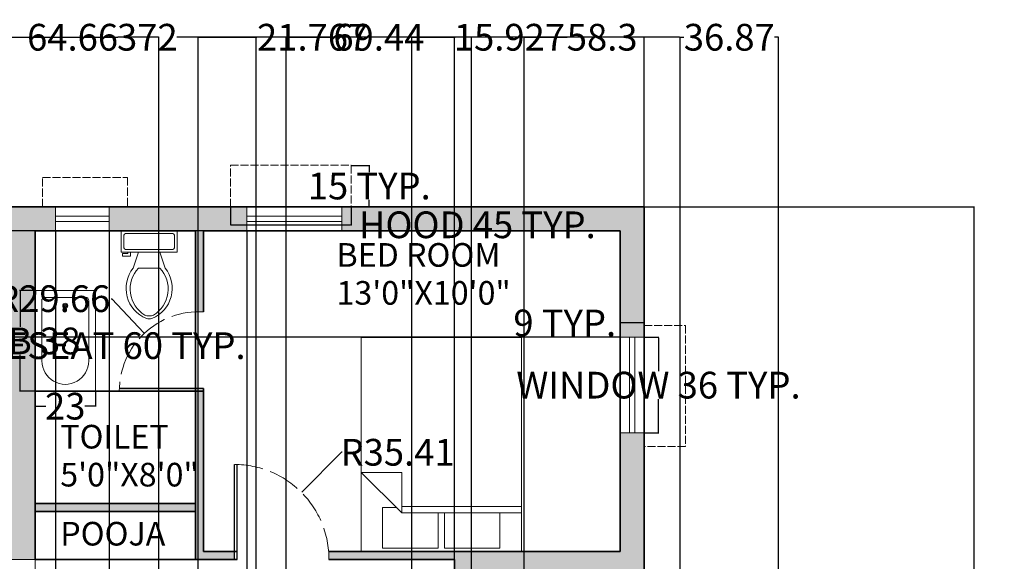
# Model space of a CAD drawing. Units: inches. Extents: x 300 to 1007, y 2 to 1069.
# Tile 12 of 12: x 617 to 986, y 867 to 1069. Entities that reach past the tile are written whole.
import ezdxf

# ---------------------------------------------------------------- set-up
doc = ezdxf.new("R2010")
doc.units = ezdxf.units.IN
doc.header["$MEASUREMENT"] = 0
doc.linetypes.add('ACAD_ISO02W100', pattern=[15, 12, -3])
for name, color, linetype, lineweight in [('A-ANNO-DIMS', 2, 'Continuous', 18), ('A-AREA-IDEN', 7, 'Continuous', 18), ('A-DOOR', 3, 'Continuous', 25), ('A-DOOR-SWNG', 3, 'ACAD_ISO02W100', 13), ('A-FLOR-FIXT', 9, 'Continuous', 18), ('A-FURN', 8, 'Continuous', 18), ('A-GLAZ', 4, 'Continuous', 18), ('A-GLAZ-OVHD', 8, 'ACAD_ISO02W100', 13), ('A-WALL', 7, 'Continuous', 35), ('A-WALL-OVHD', 8, 'ACAD_ISO02W100', 18)]:
    doc.layers.add(name, color=color, linetype=linetype, lineweight=lineweight)
doc.layers.add('A-WALL-PATT', color=9, linetype='Continuous', lineweight=9, true_color=0xc7c8ca)
doc.styles.get("Standard").update_dxf_attribs({"font": 'arial.ttf'})
doc.dimstyles.get("Standard").update_dxf_attribs({"dimtxt": 10, "dimasz": 0.18, "dimexe": 0.18, "dimexo": 0.0625, "dimgap": 0.09, "dimtad": 0, "dimtih": 1, "dimtoh": 1, "dimdec": 0, "dimzin": 0, "dimdsep": 46, "dimlunit": 3, "dimtxsty": 'Standard', "dimcen": 0.09, "dimadec": 0, "dimazin": 0, "dimtfac": 1, "dimtdec": 0, "dimtofl": 0, "dimtmove": 0, "dimatfit": 3, "dimfxl": 1, "dimtolj": 1, "dimtzin": 0, "dimarcsym": 0})

# ---------------------------------------------------------------- blocks, each defined once
blk = doc.blocks.new('Bath Tub - 26 x 60 in.')
for p, q in [((9, -17), (9, -19)), ((8, -18), (10, -18))]:
    blk.add_line(p, q)
blk.add_lwpolyline([(0, -36), (0, 0), (60, 0), (60, -36)], close=True)
for points in [[(6, -4), (42, -4)], [(4, -30), (4, -6)], [(42, -32), (6, -32)]]:
    blk.add_lwpolyline(points)
for radius in [1.5, 1]:
    blk.add_circle((9, -18), radius)
for centre, radius, start, end in [((5.75, -5.75), 1.77, 81.8699, 188.1301), ((42, -18), 14, 270, 90), ((5.75, -30.25), 1.77, 171.8699, 278.1301)]:
    blk.add_arc(centre, radius, start, end)
blk = doc.blocks.new('Toilet - top')
for p, q in [((9.5, -6), (9.5, -2)), ((-10, -8.5), (-8, -8.5)), ((-10, -9.5), (-10, -8.5)), ((-7, -9.5), (-10, -9.5)), ((-8, -8.5), (-8, -8)), ((-7, -8), (-7, -9.5)), ((-4, -8), (-6, -14)), ((4, -8), (6, -14)), ((4, -14), (-4, -14))]:
    blk.add_line(p, q)
blk.add_lwpolyline([(10.5, -8), (10.5, 0), (-10.5, 0), (-10.5, -8)], close=True)
for points in [[(-9.5, -2), (-9.5, -6)], [(8.5, -1), (-8.5, -1)], [(-8.5, -7), (8.5, -7)]]:
    blk.add_lwpolyline(points)
for centre, radius, start, end in [((-8.62, -1.88), 0.884, 81.8699, 188.1301), ((8.62, -1.88), 0.884, 351.8699, 98.1301), ((-8.62, -6.12), 0.884, 171.8699, 278.1301), ((8.62, -6.12), 0.884, 261.8699, 8.1301), ((3.52, -21.58), 12.17, 141.4691, 247.9714), ((4.2, -21.82), 11.33, 136.3677, 238.9468), ((-3.52, -21.58), 12.17, 292.0284, 38.5307), ((-4.2, -21.82), 11.33, 301.053, 43.6321), ((0, -27.88), 4, 245.7318, 294.2682), ((0, -29), 4, 254.8605, 285.1395)]:
    blk.add_arc(centre, radius, start, end)
blk = doc.blocks.new('Bed - Queen')
for p, q in [((0, -80.00003), (0, 0)), ((0, 0), (59.99999, 0)), ((59.99999, 0), (59.99999, -80.00003)), ((7.99999, -1.2), (28.79998, -1.2)), ((7.99999, -14.4), (7.99999, -1.2)), ((28.79998, -1.2), (28.79998, -14.4)), ((31.19999, -1.2), (51.99999, -1.2)), ((31.19999, -14.4), (31.19999, -1.2)), ((51.99999, -1.2), (51.99999, -16.4)), ((0, -14.4), (44.8, -14.4)), ((59.99999, -29.6), (44.8, -14.4)), ((44.8, -14.4), (44.8, -29.6)), ((44.8, -16.8), (0, -16.8)), ((51.99999, -16.4), (46.79936, -16.4)), ((44.8, -29.6), (59.99999, -29.6)), ((59.99999, -80.00003), (0, -80.00003))]:
    blk.add_line(p, q)
blk = doc.blocks.new('WIN-36')
for p, q in [((-36, -4.5), (-36, 4.5)), ((0, -4.5), (0, 4.5)), ((0, 1), (-36, 1)), ((-36, 0), (-36, -4.5)), ((0, -1), (-36, -1))]:
    blk.add_line(p, q)
blk = doc.blocks.new('WIN-35_1-2')
for p, q in [((0, -4.5), (0, 4.5)), ((35.5, 0), (35.5, 4.5)), ((35.5, 4.5), (35.5, -4.5)), ((0, 1), (35.5, 1)), ((0, -1), (35.5, -1))]:
    blk.add_line(p, q)
blk = doc.blocks.new('WINDOW-HOOD-45')
at = {"ltscale": 0.25}
for p, q in [((0, 0), (0, 15.48)), ((0, 15.48), (45.18, 15.48)), ((45.18, 15.48), (45.18, 0))]:
    blk.add_line(p, q, dxfattribs=at)
blk = doc.blocks.new('*D39')
at = {"layer": 'A-ANNO-DIMS', "color": 0, "lineweight": -2, "transparency": 16777216}
for p, q in [((622.76, 968.04), (617.01, 968.04)), ((617.19, 967.86), (617.19, 954.44)), ((617.19, 930.63), (617.19, 944.04)), ((622.76, 930.45), (617.01, 930.45))]:
    blk.add_line(p, q, dxfattribs=at)
at = {"layer": 'A-ANNO-DIMS', "color": 0, "transparency": 16777216}
for points in [[(617.16, 967.86), (617.22, 967.86), (617.19, 968.04)], [(617.16, 930.63), (617.22, 930.63), (617.19, 930.45)]]:
    blk.add_solid(points, dxfattribs=at)
at = {"layer": 'Defpoints', "color": 0, "transparency": 16777216}
for p in [(622.83, 968.04), (617.19, 930.45), (622.83, 930.45)]:
    blk.add_point(p, dxfattribs=at)
at = {"layer": 'A-ANNO-DIMS', "color": 0, "transparency": 16777216, "insert": (617.19, 949.24), "char_height": 10, "attachment_point": 5}
blk.add_mtext('\\A1;TUB 38', dxfattribs=at)
blk = doc.blocks.new('*D40')
at = {"layer": 'A-ANNO-DIMS', "color": 0, "lineweight": -2, "transparency": 16777216}
for p, q in [((622.83, 930.38), (622.83, 924.63)), ((645.38, 930.38), (645.38, 924.63)), ((623.01, 924.81), (626.77, 924.81)), ((645.2, 924.81), (641.44, 924.81))]:
    blk.add_line(p, q, dxfattribs=at)
at = {"layer": 'A-ANNO-DIMS', "color": 0, "transparency": 16777216}
for points in [[(623.01, 924.84), (623.01, 924.78), (622.83, 924.81)], [(645.2, 924.84), (645.2, 924.78), (645.38, 924.81)]]:
    blk.add_solid(points, dxfattribs=at)
at = {"layer": 'Defpoints', "color": 0, "transparency": 16777216}
for p in [(622.83, 930.45), (645.38, 930.45), (645.38, 924.81)]:
    blk.add_point(p, dxfattribs=at)
at = {"layer": 'A-ANNO-DIMS', "color": 0, "transparency": 16777216, "insert": (634.1, 924.81), "char_height": 10, "attachment_point": 5}
blk.add_mtext('\\A1;23', dxfattribs=at)
blk = doc.blocks.new('*D45')
at = {"layer": 'A-ANNO-DIMS', "color": 0, "lineweight": -2, "transparency": 16777216}
for p, q in [((850.89, 950.57), (856.37, 950.57)), ((856.19, 950.39), (856.19, 937.94)), ((856.19, 914.97), (856.19, 927.41)), ((850.89, 914.79), (856.37, 914.79))]:
    blk.add_line(p, q, dxfattribs=at)
at = {"layer": 'A-ANNO-DIMS', "color": 0, "transparency": 16777216}
for points in [[(856.16, 950.39), (856.22, 950.39), (856.19, 950.57)], [(856.16, 914.97), (856.22, 914.97), (856.19, 914.79)]]:
    blk.add_solid(points, dxfattribs=at)
at = {"layer": 'Defpoints', "color": 0, "transparency": 16777216}
for p in [(850.83, 950.57), (856.19, 950.57), (850.83, 914.79)]:
    blk.add_point(p, dxfattribs=at)
at = {"layer": 'A-ANNO-DIMS', "color": 0, "transparency": 16777216, "insert": (856.19, 932.68), "char_height": 10, "attachment_point": 5}
blk.add_mtext('\\A1;WINDOW 36 TYP.', dxfattribs=at)
blk = doc.blocks.new('*D46')
at = {"layer": 'A-ANNO-DIMS', "color": 0, "lineweight": -2, "transparency": 16777216}
for p, q in [((841.83, 955.94), (841.65, 955.94)), ((841.83, 950.63), (841.83, 956.12)), ((850.65, 955.94), (842.01, 955.94)), ((850.83, 950.63), (850.83, 956.12))]:
    blk.add_line(p, q, dxfattribs=at)
at = {"layer": 'A-ANNO-DIMS', "color": 0, "transparency": 16777216}
for points in [[(842.01, 955.97), (842.01, 955.91), (841.83, 955.94)], [(850.65, 955.97), (850.65, 955.91), (850.83, 955.94)]]:
    blk.add_solid(points, dxfattribs=at)
at = {"layer": 'Defpoints', "color": 0, "transparency": 16777216}
for p in [(841.83, 955.94), (841.83, 950.57), (850.83, 950.57)]:
    blk.add_point(p, dxfattribs=at)
at = {"layer": 'A-ANNO-DIMS', "color": 0, "transparency": 16777216, "insert": (821.1, 955.94), "char_height": 10, "attachment_point": 5}
blk.add_mtext('\\A1;9 TYP.', dxfattribs=at)
blk = doc.blocks.new('*D47')
at = {"layer": 'A-ANNO-DIMS', "color": 0, "lineweight": -2, "transparency": 16777216}
for p, q in [((695.95, 999.38), (695.95, 992.49)), ((741.12, 999.38), (741.12, 992.49)), ((696.13, 992.67), (740.94, 992.67)), ((741.12, 992.67), (741.3, 992.67))]:
    blk.add_line(p, q, dxfattribs=at)
at = {"layer": 'A-ANNO-DIMS', "color": 0, "transparency": 16777216}
for points in [[(696.13, 992.7), (696.13, 992.64), (695.95, 992.67)], [(740.94, 992.7), (740.94, 992.64), (741.12, 992.67)]]:
    blk.add_solid(points, dxfattribs=at)
at = {"layer": 'Defpoints', "color": 0, "transparency": 16777216}
for p in [(695.95, 999.45), (741.12, 999.45), (741.12, 992.67)]:
    blk.add_point(p, dxfattribs=at)
at = {"layer": 'A-ANNO-DIMS', "color": 0, "transparency": 16777216, "insert": (788.36, 992.67), "char_height": 10, "attachment_point": 5}
blk.add_mtext('\\A1;HOOD 45 TYP.', dxfattribs=at)
blk = doc.blocks.new('*D48')
at = {"layer": 'A-ANNO-DIMS', "color": 0, "lineweight": -2, "transparency": 16777216}
for p, q in [((741.19, 1014.92), (748.08, 1014.92)), ((747.9, 1014.74), (747.9, 1012.38)), ((741.19, 999.45), (748.08, 999.45)), ((747.9, 999.63), (747.9, 1001.99))]:
    blk.add_line(p, q, dxfattribs=at)
at = {"layer": 'A-ANNO-DIMS', "color": 0, "transparency": 16777216}
for points in [[(747.87, 1014.74), (747.93, 1014.74), (747.9, 1014.92)], [(747.87, 999.63), (747.93, 999.63), (747.9, 999.45)]]:
    blk.add_solid(points, dxfattribs=at)
at = {"layer": 'Defpoints', "color": 0, "transparency": 16777216}
for p in [(741.12, 1014.92), (747.9, 1014.92), (741.12, 999.45)]:
    blk.add_point(p, dxfattribs=at)
at = {"layer": 'A-ANNO-DIMS', "color": 0, "transparency": 16777216, "insert": (747.9, 1007.18), "char_height": 10, "attachment_point": 5}
blk.add_mtext('\\A1;15 TYP.', dxfattribs=at)
blk = doc.blocks.new('*D49')
at = {"layer": 'A-ANNO-DIMS', "color": 0, "lineweight": -2, "transparency": 16777216}
for p, q in [((520.83, 956.38), (520.83, 947.27)), ((580.83, 956.38), (580.83, 947.27)), ((521.01, 947.45), (580.65, 947.45)), ((580.83, 947.45), (581.01, 947.45))]:
    blk.add_line(p, q, dxfattribs=at)
at = {"layer": 'A-ANNO-DIMS', "color": 0, "transparency": 16777216}
for points in [[(521.01, 947.48), (521.01, 947.42), (520.83, 947.45)], [(580.65, 947.48), (580.65, 947.42), (580.83, 947.45)]]:
    blk.add_solid(points, dxfattribs=at)
at = {"layer": 'Defpoints', "color": 0, "transparency": 16777216}
for p in [(520.83, 956.45), (580.83, 956.45), (580.83, 947.45)]:
    blk.add_point(p, dxfattribs=at)
at = {"layer": 'A-ANNO-DIMS', "color": 0, "transparency": 16777216, "insert": (644.03, 947.45), "char_height": 10, "attachment_point": 5}
blk.add_mtext('\\A1;LOVESEAT 60 TYP.', dxfattribs=at)
blk = doc.blocks.new('*D75')
at = {"layer": 'A-ANNO-DIMS', "color": 0, "lineweight": -2, "transparency": 16777216}
for p, q in [((478.83, 999.51), (478.83, 1063.03)), ((479.01, 1062.85), (653.74, 1062.85)), ((850.65, 1062.85), (675.91, 1062.85)), ((850.83, 999.51), (850.83, 1063.03))]:
    blk.add_line(p, q, dxfattribs=at)
at = {"layer": 'A-ANNO-DIMS', "color": 0, "transparency": 16777216}
for points in [[(479.01, 1062.88), (479.01, 1062.82), (478.83, 1062.85)], [(850.65, 1062.88), (850.65, 1062.82), (850.83, 1062.85)]]:
    blk.add_solid(points, dxfattribs=at)
at = {"layer": 'Defpoints', "color": 0, "transparency": 16777216}
for p in [(850.83, 1062.85), (478.83, 999.45), (850.83, 999.45)]:
    blk.add_point(p, dxfattribs=at)
at = {"layer": 'A-ANNO-DIMS', "color": 0, "transparency": 16777216, "insert": (664.83, 1062.85), "char_height": 10, "attachment_point": 5}
blk.add_mtext('\\A1;372', dxfattribs=at)
blk = doc.blocks.new('*D78')
at = {"layer": 'A-ANNO-DIMS', "color": 0, "lineweight": -2, "transparency": 16777216}
for p, q in [((850.89, 999.45), (974.48, 999.45)), ((974.3, 999.27), (974.3, 809.65)), ((974.3, 609.63), (974.3, 799.25)), ((841.89, 609.45), (974.48, 609.45))]:
    blk.add_line(p, q, dxfattribs=at)
at = {"layer": 'A-ANNO-DIMS', "color": 0, "transparency": 16777216}
for points in [[(974.27, 999.27), (974.33, 999.27), (974.3, 999.45)], [(974.27, 609.63), (974.33, 609.63), (974.3, 609.45)]]:
    blk.add_solid(points, dxfattribs=at)
at = {"layer": 'Defpoints', "color": 0, "transparency": 16777216}
for p in [(850.83, 999.45), (974.3, 999.45), (841.83, 609.45)]:
    blk.add_point(p, dxfattribs=at)
at = {"layer": 'A-ANNO-DIMS', "color": 0, "transparency": 16777216, "insert": (974.3, 804.45), "char_height": 10, "attachment_point": 5}
blk.add_mtext('\\A1;390', dxfattribs=at)
blk = doc.blocks.new('*D80')
at = {"layer": 'A-ANNO-DIMS', "color": 0, "lineweight": -2, "transparency": 16777216}
for p, q in [((683.83, 717.31), (683.83, 1063.03)), ((684.01, 1062.85), (705.41, 1062.85)), ((705.59, 717.31), (705.59, 1063.03)), ((705.59, 1062.85), (705.77, 1062.85))]:
    blk.add_line(p, q, dxfattribs=at)
at = {"layer": 'A-ANNO-DIMS', "color": 0, "transparency": 16777216}
for points in [[(684.01, 1062.88), (684.01, 1062.82), (683.83, 1062.85)], [(705.41, 1062.88), (705.41, 1062.82), (705.59, 1062.85)]]:
    blk.add_solid(points, dxfattribs=at)
at = {"layer": 'Defpoints', "color": 0, "transparency": 16777216}
for p in [(705.59, 1062.85), (683.83, 717.25), (705.59, 717.25)]:
    blk.add_point(p, dxfattribs=at)
at = {"layer": 'A-ANNO-DIMS', "color": 0, "transparency": 16777216, "insert": (726.71, 1062.85), "char_height": 10, "attachment_point": 5}
blk.add_mtext('\\A1;21.767', dxfattribs=at)
blk = doc.blocks.new('*D82')
at = {"layer": 'A-ANNO-DIMS', "color": 0, "lineweight": -2, "transparency": 16777216}
for p, q in [((763.9, 700.01), (763.9, 1063.03)), ((764.08, 1062.85), (779.65, 1062.85)), ((779.83, 700.01), (779.83, 1063.03)), ((779.83, 1062.85), (780.01, 1062.85))]:
    blk.add_line(p, q, dxfattribs=at)
at = {"layer": 'A-ANNO-DIMS', "color": 0, "transparency": 16777216}
for points in [[(764.08, 1062.88), (764.08, 1062.82), (763.9, 1062.85)], [(779.65, 1062.88), (779.65, 1062.82), (779.83, 1062.85)]]:
    blk.add_solid(points, dxfattribs=at)
at = {"layer": 'Defpoints', "color": 0, "transparency": 16777216}
for p in [(779.83, 1062.85), (763.9, 699.95), (779.83, 699.95)]:
    blk.add_point(p, dxfattribs=at)
at = {"layer": 'A-ANNO-DIMS', "color": 0, "transparency": 16777216, "insert": (800.38, 1062.85), "char_height": 10, "attachment_point": 5}
blk.add_mtext('\\A1;15.927', dxfattribs=at)
blk = doc.blocks.new('*D84')
at = {"layer": 'A-ANNO-DIMS', "color": 0, "lineweight": -2, "transparency": 16777216}
for p, q in [((864.25, 225.89), (864.25, 1063.03)), ((864.43, 1062.85), (865.73, 1062.85)), ((900.94, 1062.85), (899.65, 1062.85)), ((901.12, 225.89), (901.12, 1063.03))]:
    blk.add_line(p, q, dxfattribs=at)
at = {"layer": 'A-ANNO-DIMS', "color": 0, "transparency": 16777216}
for points in [[(864.43, 1062.88), (864.43, 1062.82), (864.25, 1062.85)], [(900.94, 1062.88), (900.94, 1062.82), (901.12, 1062.85)]]:
    blk.add_solid(points, dxfattribs=at)
at = {"layer": 'Defpoints', "color": 0, "transparency": 16777216}
for p in [(901.12, 1062.85), (864.25, 225.83), (901.12, 225.83)]:
    blk.add_point(p, dxfattribs=at)
at = {"layer": 'A-ANNO-DIMS', "color": 0, "transparency": 16777216, "insert": (882.69, 1062.85), "char_height": 10, "attachment_point": 5}
blk.add_mtext('\\A1;36.87', dxfattribs=at)
blk = doc.blocks.new('*D86')
at = {"layer": 'A-ANNO-DIMS', "color": 0, "lineweight": -2, "transparency": 16777216}
for p, q in [((805.95, 235.15), (805.95, 1063.03)), ((806.13, 1062.85), (822.02, 1062.85)), ((864.07, 1062.85), (848.18, 1062.85)), ((864.25, 235.15), (864.25, 1063.03))]:
    blk.add_line(p, q, dxfattribs=at)
at = {"layer": 'A-ANNO-DIMS', "color": 0, "transparency": 16777216}
for points in [[(806.13, 1062.88), (806.13, 1062.82), (805.95, 1062.85)], [(864.07, 1062.88), (864.07, 1062.82), (864.25, 1062.85)]]:
    blk.add_solid(points, dxfattribs=at)
at = {"layer": 'Defpoints', "color": 0, "transparency": 16777216}
for p in [(864.25, 1062.85), (805.95, 235.08), (864.25, 235.08)]:
    blk.add_point(p, dxfattribs=at)
at = {"layer": 'A-ANNO-DIMS', "color": 0, "transparency": 16777216, "insert": (835.1, 1062.85), "char_height": 10, "attachment_point": 5}
blk.add_mtext('\\A1;58.3', dxfattribs=at)
blk = doc.blocks.new('*D94')
at = {"layer": 'A-ANNO-DIMS', "color": 0, "lineweight": -2, "transparency": 16777216}
for p, q in [((841.76, 990.45), (354.19, 990.45)), ((354.37, 990.27), (354.37, 975.71)), ((354.37, 950.75), (354.37, 965.31)), ((841.76, 950.57), (354.19, 950.57))]:
    blk.add_line(p, q, dxfattribs=at)
at = {"layer": 'A-ANNO-DIMS', "color": 0, "transparency": 16777216}
for points in [[(354.34, 990.27), (354.4, 990.27), (354.37, 990.45)], [(354.34, 950.75), (354.4, 950.75), (354.37, 950.57)]]:
    blk.add_solid(points, dxfattribs=at)
at = {"layer": 'Defpoints', "color": 0, "transparency": 16777216}
for p in [(354.37, 990.45), (841.83, 990.45), (841.83, 950.57)]:
    blk.add_point(p, dxfattribs=at)
at = {"layer": 'A-ANNO-DIMS', "color": 0, "transparency": 16777216, "insert": (354.37, 970.51), "char_height": 10, "attachment_point": 5}
blk.add_mtext('\\A1;39.88', dxfattribs=at)
blk = doc.blocks.new('*D99')
at = {"layer": 'A-ANNO-DIMS', "color": 0, "lineweight": -2, "transparency": 16777216}
for p, q in [((604.49, 482.45), (604.49, 1063.03)), ((604.67, 1062.85), (619.83, 1062.85)), ((668.97, 1062.85), (653.8, 1062.85)), ((669.15, 482.45), (669.15, 1063.03))]:
    blk.add_line(p, q, dxfattribs=at)
at = {"layer": 'A-ANNO-DIMS', "color": 0, "transparency": 16777216}
for points in [[(604.67, 1062.88), (604.67, 1062.82), (604.49, 1062.85)], [(668.97, 1062.88), (668.97, 1062.82), (669.15, 1062.85)]]:
    blk.add_solid(points, dxfattribs=at)
at = {"layer": 'Defpoints', "color": 0, "transparency": 16777216}
for p in [(669.15, 1062.85), (604.49, 482.38), (669.15, 482.38)]:
    blk.add_point(p, dxfattribs=at)
at = {"layer": 'A-ANNO-DIMS', "color": 0, "transparency": 16777216, "insert": (636.82, 1062.85), "char_height": 10, "attachment_point": 5}
blk.add_mtext('\\A1;64.66', dxfattribs=at)
blk = doc.blocks.new('*D100')
at = {"layer": 'A-ANNO-DIMS', "color": 0, "lineweight": -2, "transparency": 16777216}
for p, q in [((716.78, 482.45), (716.78, 1063.03)), ((716.96, 1062.85), (734.53, 1062.85)), ((786.04, 1062.85), (768.47, 1062.85)), ((786.22, 482.45), (786.22, 1063.03))]:
    blk.add_line(p, q, dxfattribs=at)
at = {"layer": 'A-ANNO-DIMS', "color": 0, "transparency": 16777216}
for points in [[(716.96, 1062.88), (716.96, 1062.82), (716.78, 1062.85)], [(786.04, 1062.88), (786.04, 1062.82), (786.22, 1062.85)]]:
    blk.add_solid(points, dxfattribs=at)
at = {"layer": 'Defpoints', "color": 0, "transparency": 16777216}
for p in [(786.22, 1062.85), (716.78, 482.38), (786.22, 482.38)]:
    blk.add_point(p, dxfattribs=at)
at = {"layer": 'A-ANNO-DIMS', "color": 0, "transparency": 16777216, "insert": (751.5, 1062.85), "char_height": 10, "attachment_point": 5}
blk.add_mtext('\\A1;69.44', dxfattribs=at)
blk = doc.blocks.new('*D106')
at = {"layer": 'A-ANNO-DIMS', "color": 0, "lineweight": -2, "transparency": 16777216}
for p, q in [((582.11, 990.38), (582.11, 8.45)), ((630.49, 990.38), (630.49, 8.45)), ((582.29, 8.63), (589.12, 8.63)), ((630.31, 8.63), (623.47, 8.63))]:
    blk.add_line(p, q, dxfattribs=at)
at = {"layer": 'A-ANNO-DIMS', "color": 0, "transparency": 16777216}
for points in [[(582.29, 8.66), (582.29, 8.6), (582.11, 8.63)], [(630.31, 8.66), (630.31, 8.6), (630.49, 8.63)]]:
    blk.add_solid(points, dxfattribs=at)
at = {"layer": 'Defpoints', "color": 0, "transparency": 16777216}
for p in [(582.11, 990.45), (630.49, 990.45), (630.49, 8.63)]:
    blk.add_point(p, dxfattribs=at)
at = {"layer": 'A-ANNO-DIMS', "color": 0, "transparency": 16777216, "insert": (606.3, 8.63), "char_height": 10, "attachment_point": 5}
blk.add_mtext('\\A1;48.38', dxfattribs=at)
blk = doc.blocks.new('*D107')
at = {"layer": 'A-ANNO-DIMS', "color": 0, "lineweight": -2, "transparency": 16777216}
for p, q in [((630.49, 990.38), (630.49, 8.45)), ((650.47, 990.38), (650.47, 8.45)), ((630.67, 8.63), (650.29, 8.63)), ((650.47, 8.63), (650.65, 8.63))]:
    blk.add_line(p, q, dxfattribs=at)
at = {"layer": 'A-ANNO-DIMS', "color": 0, "transparency": 16777216}
for points in [[(630.67, 8.66), (630.67, 8.6), (630.49, 8.63)], [(650.29, 8.66), (650.29, 8.6), (650.47, 8.63)]]:
    blk.add_solid(points, dxfattribs=at)
at = {"layer": 'Defpoints', "color": 0, "transparency": 16777216}
for p in [(630.49, 990.45), (650.47, 990.45), (650.47, 8.63)]:
    blk.add_point(p, dxfattribs=at)
at = {"layer": 'A-ANNO-DIMS', "color": 0, "transparency": 16777216, "insert": (667.15, 8.63), "char_height": 10, "attachment_point": 5}
blk.add_mtext('\\A1;19.98', dxfattribs=at)
blk = doc.blocks.new('*D108')
at = {"layer": 'A-ANNO-DIMS', "color": 0, "lineweight": -2, "transparency": 16777216}
for p, q in [((650.47, 990.38), (650.47, 8.45)), ((702.09, 990.38), (702.09, 8.45)), ((650.65, 8.63), (659.37, 8.63)), ((701.91, 8.63), (693.19, 8.63))]:
    blk.add_line(p, q, dxfattribs=at)
at = {"layer": 'A-ANNO-DIMS', "color": 0, "transparency": 16777216}
for points in [[(650.65, 8.66), (650.65, 8.6), (650.47, 8.63)], [(701.91, 8.66), (701.91, 8.6), (702.09, 8.63)]]:
    blk.add_solid(points, dxfattribs=at)
at = {"layer": 'Defpoints', "color": 0, "transparency": 16777216}
for p in [(650.47, 990.45), (702.09, 990.45), (702.09, 8.63)]:
    blk.add_point(p, dxfattribs=at)
at = {"layer": 'A-ANNO-DIMS', "color": 0, "transparency": 16777216, "insert": (676.28, 8.63), "char_height": 10, "attachment_point": 5}
blk.add_mtext('\\A1;51.62', dxfattribs=at)
blk = doc.blocks.new('*D114')
at = {"layer": 'A-ANNO-DIMS', "color": 0, "lineweight": -2, "transparency": 16777216}
for p, q in [((737.55, 907.56), (722.63, 892.69)), ((737.73, 907.56), (737.55, 907.56)), ((697.33, 867.57), (697.51, 867.57)), ((697.42, 867.48), (697.42, 867.66))]:
    blk.add_line(p, q, dxfattribs=at)
at = {"layer": 'A-ANNO-DIMS', "color": 0, "transparency": 16777216}
blk.add_solid([(722.61, 892.71), (722.65, 892.67), (722.5, 892.57)], dxfattribs=at)
at = {"layer": 'Defpoints', "color": 0, "transparency": 16777216}
for p in [(722.5, 892.57), (697.42, 867.57)]:
    blk.add_point(p, dxfattribs=at)
at = {"layer": 'A-ANNO-DIMS', "color": 0, "transparency": 16777216, "insert": (758.51, 907.56), "char_height": 10, "attachment_point": 5}
blk.add_mtext('\\A1;R35.41', dxfattribs=at)
blk = doc.blocks.new('*D118')
at = {"layer": 'A-ANNO-DIMS', "color": 0, "lineweight": -2, "transparency": 16777216}
for p, q in [((651.31, 965.03), (651.49, 965.03)), ((651.49, 965.03), (663.55, 952.19)), ((683.9, 930.45), (684.08, 930.45)), ((683.99, 930.36), (683.99, 930.54))]:
    blk.add_line(p, q, dxfattribs=at)
at = {"layer": 'A-ANNO-DIMS', "color": 0, "transparency": 16777216}
blk.add_solid([(663.57, 952.21), (663.53, 952.17), (663.68, 952.06)], dxfattribs=at)
at = {"layer": 'Defpoints', "color": 0, "transparency": 16777216}
for p in [(663.68, 952.06), (683.99, 930.45)]:
    blk.add_point(p, dxfattribs=at)
at = {"layer": 'A-ANNO-DIMS', "color": 0, "transparency": 16777216, "insert": (629.57, 965.03), "char_height": 10, "attachment_point": 5}
blk.add_mtext('\\A1;R29.66', dxfattribs=at)

msp = doc.modelspace()

# ---------------------------------------------------------------- hatches: boundary and pattern name
at = {"layer": 'A-WALL-PATT'}
h = msp.add_hatch(color=256, dxfattribs=at)
h.dxf.hatch_style = 1
h.paths.add_polyline_path([(546.104, 999.4468), (478.8267, 999.4468), (478.8267, 869.2798, -0.06322715), (487.8267, 868.1328), (487.8267, 990.4468), (546.104, 990.4468)])
h.paths.add_polyline_path([(630.4852, 999.4468), (582.106, 999.4468), (582.106, 990.4468), (613.8267, 990.4468), (613.8267, 867.4468), (622.8267, 867.4468), (622.8267, 990.4468), (630.4852, 990.4468)])
h.paths.add_polyline_path([(702.0883, 999.4468), (650.4653, 999.4468), (650.4653, 990.4468), (682.8267, 990.4468), (682.8267, 960.0824, -0.02530575), (685.8267, 960.0478), (685.8267, 990.4468), (702.0883, 990.4468)])
h.paths.add_polyline_path([(850.8267, 999.4468), (737.5888, 999.4468), (737.5888, 990.4468), (841.8267, 990.4468), (841.8267, 950.5685), (850.8267, 950.5685)])
h.paths.add_polyline_path([(685.8267, 930.4465), (682.8267, 930.4465), (682.8267, 888.4468), (682.8267, 867.4468), (685.8267, 867.4468), (697.4169, 867.4468), (697.4169, 870.4468), (685.8267, 870.4468), (685.8267, 888.4468)])
h.paths.add_polyline_path([(682.8267, 931.4465), (654.3436, 931.4465, 0.00843109), (654.3267, 930.4465), (682.8267, 930.4465)])
h.paths.add_polyline_path([(685.8267, 931.4465), (682.8267, 931.4465), (682.8267, 930.4465), (685.8267, 930.4465)])
h.paths.add_polyline_path([(682.8267, 888.4468), (622.8267, 888.4468), (622.8267, 885.4468), (682.8267, 885.4468)])
h.paths.add_polyline_path([(850.8267, 870.4468), (850.8267, 914.7851), (841.8267, 914.7851), (841.8267, 870.4468), (732.7101, 870.4468, -0.02120595), (732.8267, 867.4468), (779.8267, 867.4468), (779.8267, 749.4468), (782.8267, 749.4468), (788.8267, 749.4468), (788.8267, 861.4468), (841.8267, 861.4468), (841.8267, 749.4468), (850.8267, 749.4468)])
h.paths.add_polyline_path([(622.8267, 810.4468), (487.8267, 810.4468), (487.8267, 833.2626), (478.8267, 833.2626), (478.8267, 609.4468), (478.8267, 482.3847), (487.8267, 482.3847), (487.8267, 801.4468), (620.8267, 801.4468), (622.8267, 801.4468)])
h.paths.add_polyline_path([(680.8267, 729.4468), (620.8267, 729.4468), (620.8267, 765.8246, -0.02111352), (617.8267, 766.0562), (617.8267, 698.7303), (620.8267, 698.7303), (620.8267, 726.4468), (680.8267, 726.4468)])
h.paths.add_polyline_path([(620.8267, 668.8122, -0.02498293), (617.8267, 668.6448), (617.8267, 618.4468), (600.3357, 618.4468), (600.3357, 609.4468), (652.9929, 609.4468), (652.9929, 618.4468), (620.8267, 618.4468)])
h.paths.add_polyline_path([(552.3393, 618.4468), (487.8267, 618.4468), (487.8267, 609.4468), (552.3393, 609.4468)], flags=17)
h.paths.add_polyline_path([(694.5763, 618.4468), (683.8267, 618.4468), (683.8267, 726.4468), (683.8267, 749.4468), (680.8267, 749.4468), (680.8267, 740.4468), (680.8267, 726.4468), (680.8267, 618.4468), (674.1573, 618.4468), (674.1573, 609.4468), (680.8267, 609.4468), (694.5763, 609.4468)])
h.paths.add_polyline_path([(850.8267, 642.8902), (841.8267, 642.8902), (841.8267, 618.4468), (782.8267, 618.4468), (782.8267, 708.0513, -0.02308839), (779.8267, 707.9092), (779.8267, 618.4468), (730.1068, 618.4468), (730.1068, 609.4468), (779.8267, 609.4468), (841.8267, 609.4468), (841.8267, 482.3847), (850.8267, 482.3847)])
h.paths.add_polyline_path([(850.8267, 749.4468), (841.8267, 749.4468), (841.8267, 705.9119), (850.8267, 705.9119)])
h.paths.add_polyline_path([(841.8267, 749.4468), (782.8267, 749.4468), (779.8267, 749.4468), (761.9959, 749.4468), (761.9959, 740.4468), (779.8267, 740.4468), (812.3267, 740.4468), (841.8267, 740.4468)])
h.paths.add_polyline_path([(669.1457, 482.3847), (604.489, 482.3847), (604.489, 473.3847), (631.1217, 473.3847), (631.1217, 436.0244, -0.02504709), (634.1217, 436.1748), (634.1217, 436.4367), (634.1217, 473.3847), (669.1457, 473.3847)], flags=17)
h.paths.add_polyline_path([(580.5305, 482.3847), (571.1217, 482.3847), (541.0813, 482.3847), (541.0813, 473.3847), (562.1217, 473.3847), (562.1217, 326.3847), (571.1217, 326.3847), (571.1217, 362.3847), (631.1217, 362.3847), (631.1217, 326.3847), (706.9024, 326.3847, -0.02105388), (706.9999, 329.3847), (634.1217, 329.3847), (634.1217, 365.3847), (634.1217, 406.1748), (631.1217, 406.1748), (631.1217, 365.3847), (571.1217, 365.3847), (571.1217, 473.3847), (580.5305, 473.3847)])
h.paths.add_polyline_path([(493.4756, 482.3847), (420.1217, 482.3847), (420.1217, 445.3134), (429.1217, 445.3134), (429.1217, 473.3847), (493.4756, 473.3847)])
h.paths.add_polyline_path([(786.2236, 482.3847), (716.7793, 482.3847), (716.7793, 473.3847), (766.1217, 473.3847), (766.1217, 329.3847), (742.5583, 329.3847), (742.5583, 326.3847), (766.1217, 326.3847), (766.1217, 316.0647), (769.1217, 316.0647), (769.1217, 326.3847), (769.1217, 473.3847), (786.2236, 473.3847)])
h.paths.add_polyline_path([(910.1217, 482.3847), (822.7166, 482.3847), (822.7166, 473.3847), (901.1217, 473.3847), (901.1217, 402.5393), (910.1217, 402.5393)])
h.paths.add_polyline_path([(910.1217, 366.1034), (901.1217, 366.1034), (901.1217, 329.3847), (814.1217, 329.3847), (814.1217, 312.5176), (817.1217, 312.5176), (817.1217, 326.3847), (901.1217, 326.3847), (901.1217, 293.0319), (910.1217, 293.0319), (910.1217, 326.3847)])
h.paths.add_polyline_path([(910.1217, 268.9355), (901.1217, 268.9355), (901.1217, 254.3847), (817.1217, 254.3847), (817.1217, 290.5411, -0.03396715), (814.1217, 290.3847), (814.1217, 254.3847), (775.1217, 254.3847), (775.1217, 281.5164), (769.1217, 281.5164), (769.1217, 292.1577), (766.1217, 292.1577), (766.1217, 254.3847), (766.1217, 220.1938), (775.5079, 220.1938), (775.5079, 251.3847), (817.1217, 251.3847), (901.1217, 251.3847), (901.1217, 152.3847), (819.0246, 152.3847, -0.02493798), (818.9117, 149.3847), (901.1217, 149.3847), (901.1217, 92.3847), (901.1217, 83.3847), (874.3528, 83.3847), (874.3528, 74.3847), (910.1217, 74.3847), (910.1217, 92.3847), (910.1217, 149.3847)])
h.paths.add_polyline_path([(429.1217, 325.0924), (420.1217, 325.0924), (420.1217, 263.3847), (420.1217, 244.9834), (429.1217, 244.9834), (429.1217, 269.3847), (571.1217, 269.3847), (571.1217, 272.3847), (562.1217, 272.3847), (429.1217, 272.3847)])
h.paths.add_polyline_path([(429.1217, 208.998), (420.1217, 208.998), (420.1217, 74.3847), (496.7704, 74.3847), (496.7704, 83.3847), (429.1217, 83.3847)])
h.paths.add_polyline_path([(598.4322, 83.3847), (571.1217, 83.3847), (571.1217, 122.1171), (562.1217, 122.1171), (562.1217, 83.3847), (544.6031, 83.3847), (544.6031, 74.3847), (598.4322, 74.3847)])
h.paths.add_polyline_path([(797.0822, 83.3847), (769.1217, 83.3847), (769.1217, 149.3847), (788.9123, 149.3847), (788.9123, 152.3847), (769.1217, 152.3847), (769.1217, 178.0167), (766.1217, 178.0167), (766.1217, 152.3847), (735.3598, 152.3847), (735.3598, 143.3847), (766.1217, 143.3847), (766.1217, 83.3847), (634.1217, 83.3847), (634.1217, 143.3847), (659.7326, 143.3847), (659.7326, 152.3847), (634.1217, 152.3847), (634.1217, 194.3847), (571.1217, 194.3847), (571.1217, 233.7289, -0.06379947), (562.1217, 234.7942), (562.1217, 163.4485), (567.7403, 163.4485), (567.7403, 152.3847), (571.1217, 152.3847), (571.1217, 191.3847), (631.1217, 191.3847), (631.1217, 83.3847), (621.979, 83.3847), (621.979, 74.3847), (631.1217, 74.3847), (797.0822, 74.3847)])

# ---------------------------------------------------------------- linework, layer by layer
at = {"layer": 'A-DOOR'}
for p, q in [((685.8267, 960.0478), (685.8267, 960.0478)), ((685.8267, 931.4465), (654.3267, 931.4465)), ((685.8267, 930.4465), (654.3267, 930.4465)), ((685.8267, 930.4465), (685.8267, 931.4465)), ((697.4169, 867.4468), (697.4169, 902.9822)), ((698.4169, 867.4468), (698.4169, 902.9822)), ((697.4169, 867.4468), (697.4169, 870.4468)), ((697.4169, 867.4468), (698.4169, 867.4468))]:
    msp.add_line(p, q, dxfattribs=at)
at = {"layer": 'A-DOOR-SWNG'}
for centre, radius, start, end in [((683.9852, 930.4465), 29.6585, 86.440183, 180), ((697.4169, 867.5722), 35.4101, 359.797136, 90)]:
    msp.add_arc(centre, radius, start, end, dxfattribs=at)
at = {"layer": 'A-GLAZ'}
for p, q in [((630.4852, 990.4468), (630.4852, 999.4468)), ((650.4653, 994.9468), (650.4653, 999.4468)), ((650.4653, 999.4468), (650.4653, 990.4468)), ((630.4852, 995.9468), (650.4653, 995.9468)), ((630.4852, 993.9468), (650.4653, 993.9468))]:
    msp.add_line(p, q, dxfattribs=at)
at = {"layer": 'A-GLAZ-OVHD', "ltscale": 0.25}
for p, q in [((625.5853, 999.4468), (625.5853, 1010.3215)), ((625.5853, 1010.3215), (657.3318, 1010.3215)), ((657.3318, 1010.3215), (657.3318, 999.4468))]:
    msp.add_line(p, q, dxfattribs=at)
at = {"layer": 'A-WALL'}
for p, q in [((478.8267, 999.4468), (850.8267, 999.4468)), ((622.8267, 999.4468), (682.8267, 999.4468)), ((850.8267, 999.4468), (850.8267, 870.4468)), ((622.8267, 867.4468), (622.8267, 990.4468)), ((622.8267, 990.4468), (682.8267, 990.4468)), ((682.8267, 990.4468), (682.8267, 888.4468)), ((685.8267, 990.4468), (685.8267, 960.0478)), ((685.8267, 990.4468), (841.8267, 990.4468)), ((841.8267, 990.4468), (841.8267, 870.4468)), ((685.8267, 930.4465), (622.8267, 930.4465)), ((685.8267, 931.4465), (685.8267, 888.4468)), ((682.8267, 888.4468), (622.8267, 888.4468)), ((682.8267, 867.4468), (682.8267, 888.4468)), ((685.8267, 870.4468), (685.8267, 888.4468)), ((682.8267, 885.4468), (622.8267, 885.4468)), ((698.4169, 870.4468), (685.8267, 870.4468)), ((841.8267, 870.4468), (732.7101, 870.4468)), ((850.8267, 749.4468), (850.8267, 870.4468)), ((685.8267, 867.4468), (622.8267, 867.4468)), ((698.4169, 867.4468), (685.8267, 867.4468)), ((779.8267, 867.4468), (732.8267, 867.4468)), ((779.8267, 749.4468), (779.8267, 867.4468))]:
    msp.add_line(p, q, dxfattribs=at)
at = {"layer": 'A-WALL-OVHD'}
for q in [(613.8267, 867.4468), (622.8267, 810.4468)]:
    msp.add_line((622.8267, 867.4468), q, dxfattribs=at)

# ---------------------------------------------------------------- block references
at = {"layer": 'A-FLOR-FIXT'}
msp.add_blockref('Toilet - top', (665.4877, 990.4468), dxfattribs=at)
at = {"layer": 'A-FLOR-FIXT', "xscale": 0.6264982043070834, "yscale": 0.6264982043070834, "zscale": 0.6264982043070834, "rotation": 270}
msp.add_blockref('Bath Tub - 26 x 60 in.', (645.3806, 968.0364), dxfattribs=at)
at = {"layer": 'A-FURN', "rotation": 180}
msp.add_blockref('Bed - Queen', (804.8396, 870.4468), dxfattribs=at)
at = {"layer": 'A-GLAZ'}
msp.add_blockref('WIN-35_1-2', (702.0883, 994.9468), dxfattribs=at)
at = {"layer": 'A-GLAZ', "xscale": 0.993927254948014, "rotation": 90}
msp.add_blockref('WIN-36', (846.3267, 950.5685), dxfattribs=at)
at = {"layer": 'A-GLAZ-OVHD'}
msp.add_blockref('WINDOW-HOOD-45', (695.9485, 999.4468), dxfattribs=at)
at = {"layer": 'A-GLAZ-OVHD', "rotation": 270.0000000000001}
msp.add_blockref('WINDOW-HOOD-45', (850.8267, 954.9553), dxfattribs=at)

# ---------------------------------------------------------------- texts
at = {"layer": 'A-AREA-IDEN'}
for s, height, p in [('BED ROOM ', 8.8435, (735.6372, 976.9813)), ('13\'0"X10\'0"', 8.843498, (735.6372, 962.775)), ('TOILET', 8.8435, (632.2155, 908.9713)), ('5\'0"X8\'0"', 8.8435, (632.2155, 894.765)), ('POOJA', 8.8435, (632.2155, 872.6706))]:
    msp.add_text(s, height=height, dxfattribs=at).set_placement(p)

# ---------------------------------------------------------------- dimensions: what is measured, and where the dimension line sits
at = {"layer": 'A-ANNO-DIMS'}
for base, p1, p2, override, picture, middle in [((850.8267, 1062.8469), (478.8267, 999.4468), (850.8267, 999.4468), {"dimdec": 0, "dimlfac": 1, "dimrnd": 0, "dimzin": 0, "dimdsep": 46, "dimlunit": 2}, '*D75', (664.8267, 1062.8469)), ((669.1457, 1062.8469), (604.489, 482.3847), (669.1457, 482.3847), {"dimdec": 2, "dimlfac": 1, "dimrnd": 0, "dimzin": 0, "dimdsep": 46, "dimlunit": 2}, '*D99', (636.8174, 1062.8469)), ((705.5939, 1062.8469), (683.8267, 717.2516), (705.5939, 717.2516), {"dimdec": 3, "dimlfac": 1, "dimrnd": 0, "dimzin": 0, "dimdsep": 46, "dimlunit": 2}, '*D80', (726.7063, 1062.8469)), ((786.2236, 1062.8469), (716.7793, 482.3847), (786.2236, 482.3847), {"dimdec": 2, "dimlfac": 1, "dimrnd": 0, "dimzin": 0, "dimdsep": 46, "dimlunit": 2}, '*D100', (751.5015, 1062.8469)), ((779.8267, 1062.8469), (763.9001, 699.9453), (779.8267, 699.9453), {"dimdec": 3, "dimlfac": 1, "dimrnd": 0, "dimzin": 0, "dimdsep": 46, "dimlunit": 2}, '*D82', (800.3832, 1062.8469)), ((864.2528, 1062.8469), (805.95, 235.0834), (864.2528, 235.0834), {"dimdec": 1, "dimlfac": 1, "dimrnd": 0, "dimzin": 0, "dimdsep": 46, "dimlunit": 2}, '*D86', (835.1014, 1062.8469)), ((901.1217, 1062.8469), (864.2528, 225.8264), (901.1217, 225.8264), {"dimdec": 2, "dimlfac": 1, "dimrnd": 0, "dimzin": 0, "dimdsep": 46, "dimlunit": 2}, '*D84', (882.6872, 1062.8469)), ((630.4852, 8.6288), (582.106, 990.4468), (630.4852, 990.4468), {"dimdec": 2, "dimlfac": 1, "dimrnd": 0, "dimzin": 0, "dimdsep": 46, "dimlunit": 2}, '*D106', (606.2956, 8.6288)), ((650.4653, 8.6288), (630.4852, 990.4468), (650.4653, 990.4468), {"dimdec": 2, "dimlfac": 1, "dimrnd": 0, "dimzin": 0, "dimdsep": 46, "dimlunit": 2}, '*D107', (667.1473, 8.6288)), ((702.0883, 8.6288), (650.4653, 990.4468), (702.0883, 990.4468), {"dimdec": 2, "dimlfac": 1, "dimrnd": 0, "dimzin": 0, "dimdsep": 46, "dimlunit": 2}, '*D108', (676.2768, 8.6288)), ((645.3806, 924.808), (622.8267, 930.4465), (645.3806, 930.4465), {"dimdec": 0, "dimlfac": 1, "dimrnd": 0, "dimzin": 0, "dimdsep": 46, "dimlunit": 2}, '*D40', (634.1037, 924.808))]:
    dim = msp.add_linear_dim(base=base, p1=p1, p2=p2, dimstyle='Standard', override=override, dxfattribs=at)
    dim.commit()
    dim.dimension.update_dxf_attribs({"geometry": picture, "text_midpoint": middle})
for base, p1, p2, angle, text, picture, middle in [((747.9012, 1014.9219), (741.1248, 999.4468), (741.1248, 1014.9219), 90, '<> TYP.', '*D48', (747.9012, 1007.1844)), ((841.8267, 955.936), (850.8267, 950.5685), (841.8267, 950.5685), 180, '<> TYP.', '*D46', (821.1031, 955.936)), ((617.1882, 930.4465), (622.8267, 968.0364), (622.8267, 930.4465), 270, 'TUB <>', '*D39', (617.1882, 949.2415)), ((856.1942, 950.5685), (850.8267, 914.7851), (850.8267, 950.5685), 90, 'WINDOW <> TYP.', '*D45', (856.1942, 932.6768))]:
    dim = msp.add_linear_dim(base=base, p1=p1, p2=p2, angle=angle, text=text, dimstyle='Standard', override={"dimdec": 0, "dimlfac": 1, "dimrnd": 0, "dimzin": 0, "dimdsep": 46, "dimlunit": 2}, dxfattribs=at)
    dim.commit()
    dim.dimension.update_dxf_attribs({"geometry": picture, "text_midpoint": middle})
for base, p1, p2, text, picture, middle in [((741.1248, 992.6703), (695.9485, 999.4468), (741.1248, 999.4468), 'HOOD <> TYP.', '*D47', (788.3593, 992.6703)), ((580.8267, 947.4468), (520.8267, 956.4468), (580.8267, 956.4468), 'LOVESEAT <> TYP.', '*D49', (644.0333, 947.4468))]:
    dim = msp.add_linear_dim(base=base, p1=p1, p2=p2, text=text, dimstyle='Standard', override={"dimdec": 0, "dimlfac": 1, "dimrnd": 0, "dimzin": 0, "dimdsep": 46, "dimlunit": 2}, dxfattribs=at)
    dim.commit()
    dim.dimension.update_dxf_attribs({"geometry": picture, "text_midpoint": middle})
for base, p1, p2, override, picture, middle in [((974.3023, 999.4468), (841.8267, 609.4468), (850.8267, 999.4468), {"dimdec": 0, "dimlfac": 1, "dimrnd": 0, "dimzin": 0, "dimdsep": 46, "dimlunit": 2}, '*D78', (974.3023, 804.4468)), ((354.3658, 990.4468), (841.8267, 950.5685), (841.8267, 990.4468), {"dimdec": 2, "dimlfac": 1, "dimrnd": 0, "dimzin": 0, "dimdsep": 46, "dimlunit": 2}, '*D94', (354.3658, 970.5076))]:
    dim = msp.add_linear_dim(base=base, p1=p1, p2=p2, angle=90, dimstyle='Standard', override=override, dxfattribs=at)
    dim.commit()
    dim.dimension.update_dxf_attribs({"geometry": picture, "text_midpoint": middle})
for center, mpoint, picture, middle in [((683.9852, 930.4465), (663.6752, 952.0598), '*D118', (629.5651, 965.0277)), ((697.4169, 867.5722), (722.5002, 892.5662), '*D114', (758.5125, 907.5626))]:
    dim = msp.add_radius_dim(center=center, mpoint=mpoint, dimstyle='Standard', override={"dimdec": 2, "dimlfac": 1, "dimrnd": 0, "dimzin": 0, "dimdsep": 46, "dimlunit": 2}, dxfattribs=at)
    dim.commit()
    dim.dimension.update_dxf_attribs({"geometry": picture, "text_midpoint": middle, "dimtype": 164})

doc.saveas('drawing.dxf')
